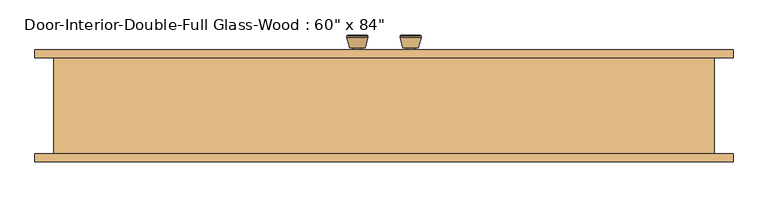
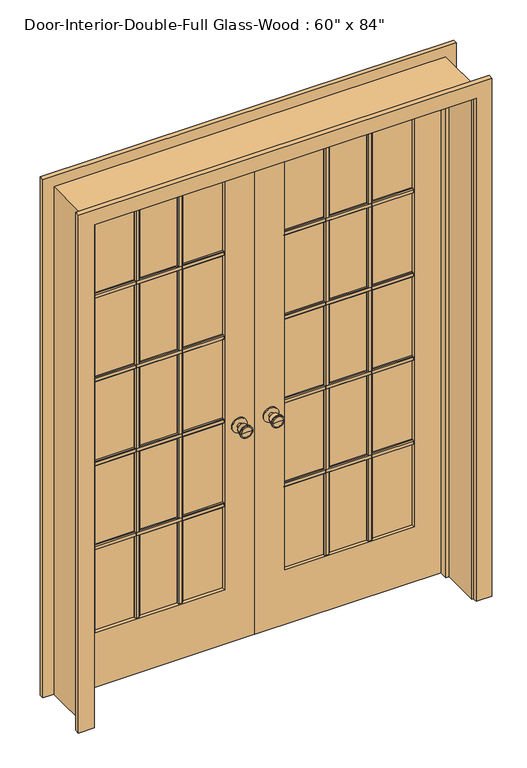
"""IFC4 building model written with IfcOpenShell, lengths in millimetres: door geometry."""

from ifc_helpers import new_model, si_unit, point, frame, frame_2d, origin, place, context, project, spatial, polyline, circle_curve, trimmed, segment, composite_curve, outline, extrude, faceted_brep, source, transform, mapped, element, save
from ifc_brep_helpers import plane_surface, cylinder_surface, revolved_surface, advanced_brep


def door_610bc5f6(model_context):
    return source(origin(), model_context, "Body", "SolidModel", [
        advanced_brep(
        [(-63.5, 117.125, 914.4), (-73.5, 117.125, 914.4), (-53.5, 117.125, 914.4), (-83.9758676, 166.125, 914.4), (-63.5, 166.125, 914.4), (-43.0241324, 166.125, 914.4), (-88.5, 164.2971319, 914.4), (-38.5, 164.2971319, 914.4), (-88.5, 160.8334537, 914.4), (-38.5, 160.8334537, 914.4), (-82.136236, 136.125, 914.4), (-44.863764, 136.125, 914.4), (-73.5, 136.125, 914.4), (-53.5, 136.125, 914.4)],
        [
            (0, 1),
            (1, 2, circle_curve(frame((-63.5, 117.125, 914.4), z_axis=(0.0, -1.0, 0.0), x_axis=(1.0, 0.0, 0.0)), 10.0)),
            (2, 0),
            (2, 1, circle_curve(frame((-63.5, 117.125, 914.4), z_axis=(0.0, -1.0, 0.0), x_axis=(1.0, 0.0, 0.0)), 10.0)),
            (3, 4),
            (4, 5),
            (5, 3, circle_curve(frame((-63.5, 166.125, 914.4), z_axis=(0.0, 1.0, 0.0), x_axis=(1.0, 0.0, 0.0)), 20.4758676)),
            (3, 5, circle_curve(frame((-63.5, 166.125, 914.4), z_axis=(0.0, 1.0, 0.0), x_axis=(1.0, 0.0, 0.0)), 20.4758676)),
            (6, 3),
            (5, 7),
            (7, 6, circle_curve(frame((-63.5, 164.2971319, 914.4), z_axis=(0.0, 1.0, 0.0), x_axis=(1.0, 0.0, 0.0)), 25.0)),
            (6, 7, circle_curve(frame((-63.5, 164.2971319, 914.4), z_axis=(0.0, 1.0, 0.0), x_axis=(1.0, 0.0, 0.0)), 25.0)),
            (8, 6),
            (7, 9),
            (9, 8, circle_curve(frame((-63.5, 160.8334537, 914.4), z_axis=(0.0, 1.0, 0.0), x_axis=(1.0, 0.0, 0.0)), 25.0)),
            (8, 9, circle_curve(frame((-63.5, 160.8334537, 914.4), z_axis=(0.0, 1.0, 0.0), x_axis=(1.0, 0.0, 0.0)), 25.0)),
            (10, 8),
            (9, 11),
            (11, 10, circle_curve(frame((-63.5, 136.125, 914.4), z_axis=(0.0, 1.0, 0.0), x_axis=(1.0, 0.0, 0.0)), 18.636236)),
            (10, 11, circle_curve(frame((-63.5, 136.125, 914.4), z_axis=(0.0, 1.0, 0.0), x_axis=(1.0, 0.0, 0.0)), 18.636236)),
            (12, 10),
            (11, 13),
            (13, 12, circle_curve(frame((-63.5, 136.125, 914.4), z_axis=(0.0, 1.0, 0.0), x_axis=(1.0, 0.0, 0.0)), 10.0)),
            (12, 13, circle_curve(frame((-63.5, 136.125, 914.4), z_axis=(0.0, 1.0, 0.0), x_axis=(1.0, 0.0, 0.0)), 10.0)),
            (1, 12),
            (13, 2),
        ],
        [
            plane_surface(frame((-63.5, 117.125, 914.4), z_axis=(0.0, -1.0, 0.0), x_axis=(1.0, 0.0, 0.0))),
            plane_surface(frame((-63.5, 166.125, 914.4), z_axis=(0.0, 1.0, 0.0), x_axis=(1.0, 0.0, 0.0))),
            revolved_surface(polyline([(-43.0241324, 166.125, 914.4), (-38.5, 164.2971319, 914.4)]), (-63.5, 117.125, 914.4), (0.0, -1.0, 0.0)),
            cylinder_surface(frame((-63.5, 117.125, 914.4), z_axis=(0.0, -1.0, 0.0), x_axis=(1.0, 0.0, 0.0)), 25.0),
            revolved_surface(polyline([(-38.5, 160.8334537, 914.4), (-44.863764, 136.125, 914.4)]), (-63.5, 117.125, 914.4), (0.0, -1.0, 0.0)),
            plane_surface(frame((-63.5, 136.125, 914.4), z_axis=(0.0, -1.0, 0.0), x_axis=(1.0, 0.0, 0.0))),
            cylinder_surface(frame((-63.5, 117.125, 914.4), z_axis=(0.0, -1.0, 0.0), x_axis=(1.0, 0.0, 0.0)), 10.0),
        ],
        [
            (0, [[1, 2, 3]]),
            (0, [[-3, 4, -1]]),
            (1, [[5, 6, 7]]),
            (1, [[-6, -5, 8]]),
            (2, [[9, -7, 10, 11]]),
            (2, [[-10, -8, -9, 12]]),
            (3, [[13, -11, 14, 15]]),
            (3, [[-14, -12, -13, 16]]),
            (4, [[17, -15, 18, 19]]),
            (4, [[-18, -16, -17, 20]]),
            (5, [[21, -19, 22, 23]]),
            (5, [[-22, -20, -21, 24]]),
            (6, [[25, -23, 26, -2]]),
            (6, [[-26, -24, -25, -4]]),
        ],
    ),
        extrude(outline(composite_curve([segment(trimmed(circle_curve(frame_2d((914.4, -63.5)), 30.0), [point((914.4, -33.5))], [point((914.4, -93.5))], False, "CARTESIAN"), True, "CONTINUOUS"), segment(trimmed(circle_curve(frame_2d((914.4, -63.5)), 30.0), [point((914.4, -93.5))], [point((914.4, -33.5))], False, "CARTESIAN"), True, "CONTINUOUS")], self_intersect=False)), frame((0.0, 111.125, 0.0), z_axis=(0.0, 1.0, 0.0), x_axis=(0.0, 0.0, 1.0)), (0.0, 0.0, 1.0), 6.0),
        advanced_brep(
        [(-63.5, 70.2, 914.4), (-53.5, 70.2, 914.4), (-73.5, 70.2, 914.4), (-83.9758676, 21.2, 914.4), (-43.0241324, 21.2, 914.4), (-63.5, 21.2, 914.4), (-88.5, 23.0278681, 914.4), (-38.5, 23.0278681, 914.4), (-88.5, 26.4915463, 914.4), (-38.5, 26.4915463, 914.4), (-82.136236, 51.2, 914.4), (-44.863764, 51.2, 914.4), (-73.5, 51.2, 914.4), (-53.5, 51.2, 914.4)],
        [
            (0, 1),
            (1, 2, circle_curve(frame((-63.5, 70.2, 914.4), z_axis=(0.0, 1.0, 0.0), x_axis=(1.0, 0.0, 0.0)), 10.0)),
            (2, 0),
            (2, 1, circle_curve(frame((-63.5, 70.2, 914.4), z_axis=(0.0, 1.0, 0.0), x_axis=(1.0, 0.0, 0.0)), 10.0)),
            (3, 4, circle_curve(frame((-63.5, 21.2, 914.4), z_axis=(0.0, -1.0, 0.0), x_axis=(1.0, 0.0, 0.0)), 20.4758676)),
            (4, 5),
            (5, 3),
            (4, 3, circle_curve(frame((-63.5, 21.2, 914.4), z_axis=(0.0, -1.0, 0.0), x_axis=(1.0, 0.0, 0.0)), 20.4758676)),
            (6, 7, circle_curve(frame((-63.5, 23.0278681, 914.4), z_axis=(0.0, -1.0, 0.0), x_axis=(1.0, 0.0, 0.0)), 25.0)),
            (7, 4),
            (3, 6),
            (7, 6, circle_curve(frame((-63.5, 23.0278681, 914.4), z_axis=(0.0, -1.0, 0.0), x_axis=(1.0, 0.0, 0.0)), 25.0)),
            (8, 9, circle_curve(frame((-63.5, 26.4915463, 914.4), z_axis=(0.0, -1.0, 0.0), x_axis=(1.0, 0.0, 0.0)), 25.0)),
            (9, 7),
            (6, 8),
            (9, 8, circle_curve(frame((-63.5, 26.4915463, 914.4), z_axis=(0.0, -1.0, 0.0), x_axis=(1.0, 0.0, 0.0)), 25.0)),
            (10, 11, circle_curve(frame((-63.5, 51.2, 914.4), z_axis=(0.0, -1.0, 0.0), x_axis=(1.0, 0.0, 0.0)), 18.636236)),
            (11, 9),
            (8, 10),
            (11, 10, circle_curve(frame((-63.5, 51.2, 914.4), z_axis=(0.0, -1.0, 0.0), x_axis=(1.0, 0.0, 0.0)), 18.636236)),
            (12, 13, circle_curve(frame((-63.5, 51.2, 914.4), z_axis=(0.0, -1.0, 0.0), x_axis=(1.0, 0.0, 0.0)), 10.0)),
            (13, 11),
            (10, 12),
            (13, 12, circle_curve(frame((-63.5, 51.2, 914.4), z_axis=(0.0, -1.0, 0.0), x_axis=(1.0, 0.0, 0.0)), 10.0)),
            (1, 13),
            (12, 2),
        ],
        [
            plane_surface(frame((-63.5, 70.2, 914.4), z_axis=(0.0, 1.0, 0.0), x_axis=(1.0, 0.0, 0.0))),
            plane_surface(frame((-63.5, 21.2, 914.4), z_axis=(0.0, -1.0, 0.0), x_axis=(1.0, 0.0, 0.0))),
            revolved_surface(polyline([(-43.0241324, 21.2, 914.4), (-38.5, 23.0278681, 914.4)]), (-63.5, 70.2, 914.4), (0.0, 1.0, 0.0)),
            cylinder_surface(frame((-63.5, 70.2, 914.4), z_axis=(0.0, 1.0, 0.0), x_axis=(1.0, 0.0, 0.0)), 25.0),
            revolved_surface(polyline([(-38.5, 26.4915463, 914.4), (-44.863764, 51.2, 914.4)]), (-63.5, 70.2, 914.4), (0.0, 1.0, 0.0)),
            plane_surface(frame((-63.5, 51.2, 914.4), z_axis=(0.0, 1.0, 0.0), x_axis=(1.0, 0.0, 0.0))),
            cylinder_surface(frame((-63.5, 70.2, 914.4), z_axis=(0.0, 1.0, 0.0), x_axis=(1.0, 0.0, 0.0)), 10.0),
        ],
        [
            (0, [[1, 2, 3]]),
            (0, [[-3, 4, -1]]),
            (1, [[5, 6, 7]]),
            (1, [[8, -7, -6]]),
            (2, [[9, 10, -5, 11]]),
            (2, [[12, -11, -8, -10]]),
            (3, [[13, 14, -9, 15]]),
            (3, [[16, -15, -12, -14]]),
            (4, [[17, 18, -13, 19]]),
            (4, [[20, -19, -16, -18]]),
            (5, [[21, 22, -17, 23]]),
            (5, [[24, -23, -20, -22]]),
            (6, [[-2, 25, -21, 26]]),
            (6, [[-4, -26, -24, -25]]),
        ],
    ),
        extrude(outline(composite_curve([segment(trimmed(circle_curve(frame_2d((914.4, -63.5)), 30.0), [point((914.4, -33.5))], [point((914.4, -93.5))], False, "CARTESIAN"), True, "CONTINUOUS"), segment(trimmed(circle_curve(frame_2d((914.4, -63.5)), 30.0), [point((914.4, -93.5))], [point((914.4, -33.5))], False, "CARTESIAN"), True, "CONTINUOUS")], self_intersect=False)), frame((0.0, 70.2, 0.0), z_axis=(0.0, 1.0, 0.0), x_axis=(0.0, 0.0, 1.0)), (0.0, 0.0, 1.0), 6.0),
        extrude(outline(polyline([(90.17, 1667.51), (90.17, 1648.46), (83.82, 1648.46), (80.645, 1651.635), (80.645, 1664.335), (83.82, 1667.51), (90.17, 1667.51)])), frame((120.65, 0.0, 0.0), z_axis=(1.0, 0.0, 0.0), x_axis=(0.0, 1.0, 0.0)), (0.0, 0.0, 1.0), 520.7),
        extrude(outline(polyline([(90.17, 1310.9575), (90.17, 1291.9075), (83.82, 1291.9075), (80.645, 1295.0825), (80.645, 1307.7825), (83.82, 1310.9575), (90.17, 1310.9575)])), frame((120.65, 0.0, 0.0), z_axis=(1.0, 0.0, 0.0), x_axis=(0.0, 1.0, 0.0)), (0.0, 0.0, 1.0), 520.7),
        extrude(outline(polyline([(90.17, 954.405), (90.17, 935.355), (83.82, 935.355), (80.645, 938.53), (80.645, 951.23), (83.82, 954.405), (90.17, 954.405)])), frame((120.65, 0.0, 0.0), z_axis=(1.0, 0.0, 0.0), x_axis=(0.0, 1.0, 0.0)), (0.0, 0.0, 1.0), 520.7),
        extrude(outline(polyline([(90.17, 597.8525), (90.17, 578.8025), (83.82, 578.8025), (80.645, 581.9775), (80.645, 594.6775), (83.82, 597.8525), (90.17, 597.8525)])), frame((120.65, 0.0, 0.0), z_axis=(1.0, 0.0, 0.0), x_axis=(0.0, 1.0, 0.0)), (0.0, 0.0, 1.0), 520.7),
        extrude(outline(polyline([(458.2583333, 90.17), (477.3083333, 90.17), (477.3083333, 83.82), (474.1333333, 80.645), (461.4333333, 80.645), (458.2583333, 83.82), (458.2583333, 90.17)])), frame((0.0, 0.0, 231.775), z_axis=(0.0, 0.0, 1.0), x_axis=(1.0, 0.0, 0.0)), (0.0, 0.0, 1.0), 1782.7625),
        extrude(outline(polyline([(284.6916667, 90.17), (303.7416667, 90.17), (303.7416667, 83.82), (300.5666667, 80.645), (287.8666667, 80.645), (284.6916667, 83.82), (284.6916667, 90.17)])), frame((0.0, 0.0, 231.775), z_axis=(0.0, 0.0, 1.0), x_axis=(1.0, 0.0, 0.0)), (0.0, 0.0, 1.0), 1782.7625),
        extrude(outline(polyline([(97.155, 1667.51), (103.505, 1667.51), (106.68, 1664.335), (106.68, 1651.635), (103.505, 1648.46), (97.155, 1648.46), (97.155, 1667.51)])), frame((-641.35, 0.0, 0.0), z_axis=(1.0, 0.0, 0.0), x_axis=(0.0, 1.0, 0.0)), (0.0, 0.0, 1.0), 520.7),
        extrude(outline(polyline([(97.155, 1310.9575), (103.505, 1310.9575), (106.68, 1307.7825), (106.68, 1295.0825), (103.505, 1291.9075), (97.155, 1291.9075), (97.155, 1310.9575)])), frame((-641.35, 0.0, 0.0), z_axis=(1.0, 0.0, 0.0), x_axis=(0.0, 1.0, 0.0)), (0.0, 0.0, 1.0), 520.7),
        extrude(outline(polyline([(97.155, 954.405), (103.505, 954.405), (106.68, 951.23), (106.68, 938.53), (103.505, 935.355), (97.155, 935.355), (97.155, 954.405)])), frame((-641.35, 0.0, 0.0), z_axis=(1.0, 0.0, 0.0), x_axis=(0.0, 1.0, 0.0)), (0.0, 0.0, 1.0), 520.7),
        extrude(outline(polyline([(97.155, 597.8525), (103.505, 597.8525), (106.68, 594.6775), (106.68, 581.9775), (103.505, 578.8025), (97.155, 578.8025), (97.155, 597.8525)])), frame((-641.35, 0.0, 0.0), z_axis=(1.0, 0.0, 0.0), x_axis=(0.0, 1.0, 0.0)), (0.0, 0.0, 1.0), 520.7),
        extrude(outline(polyline([(-303.7416667, 97.155), (-303.7416667, 103.505), (-300.5666667, 106.68), (-287.8666667, 106.68), (-284.6916667, 103.505), (-284.6916667, 97.155), (-303.7416667, 97.155)])), frame((0.0, 0.0, 231.775), z_axis=(0.0, 0.0, 1.0), x_axis=(1.0, 0.0, 0.0)), (0.0, 0.0, 1.0), 1782.7625),
        extrude(outline(polyline([(-477.3083333, 97.155), (-477.3083333, 103.505), (-474.1333333, 106.68), (-461.4333333, 106.68), (-458.2583333, 103.505), (-458.2583333, 97.155), (-477.3083333, 97.155)])), frame((0.0, 0.0, 231.775), z_axis=(0.0, 0.0, 1.0), x_axis=(1.0, 0.0, 0.0)), (0.0, 0.0, 1.0), 1782.7625),
        extrude(outline(polyline([(97.155, 1667.51), (103.505, 1667.51), (106.68, 1664.335), (106.68, 1651.635), (103.505, 1648.46), (97.155, 1648.46), (97.155, 1667.51)])), frame((120.65, 0.0, 0.0), z_axis=(1.0, 0.0, 0.0), x_axis=(0.0, 1.0, 0.0)), (0.0, 0.0, 1.0), 520.7),
        extrude(outline(polyline([(97.155, 1310.9575), (103.505, 1310.9575), (106.68, 1307.7825), (106.68, 1295.0825), (103.505, 1291.9075), (97.155, 1291.9075), (97.155, 1310.9575)])), frame((120.65, 0.0, 0.0), z_axis=(1.0, 0.0, 0.0), x_axis=(0.0, 1.0, 0.0)), (0.0, 0.0, 1.0), 520.7),
        extrude(outline(polyline([(97.155, 954.405), (103.505, 954.405), (106.68, 951.23), (106.68, 938.53), (103.505, 935.355), (97.155, 935.355), (97.155, 954.405)])), frame((120.65, 0.0, 0.0), z_axis=(1.0, 0.0, 0.0), x_axis=(0.0, 1.0, 0.0)), (0.0, 0.0, 1.0), 520.7),
        extrude(outline(polyline([(97.155, 597.8525), (103.505, 597.8525), (106.68, 594.6775), (106.68, 581.9775), (103.505, 578.8025), (97.155, 578.8025), (97.155, 597.8525)])), frame((120.65, 0.0, 0.0), z_axis=(1.0, 0.0, 0.0), x_axis=(0.0, 1.0, 0.0)), (0.0, 0.0, 1.0), 520.7),
        extrude(outline(polyline([(458.2583333, 97.155), (458.2583333, 103.505), (461.4333333, 106.68), (474.1333333, 106.68), (477.3083333, 103.505), (477.3083333, 97.155), (458.2583333, 97.155)])), frame((0.0, 0.0, 231.775), z_axis=(0.0, 0.0, 1.0), x_axis=(1.0, 0.0, 0.0)), (0.0, 0.0, 1.0), 1782.7625),
        extrude(outline(polyline([(284.6916667, 97.155), (284.6916667, 103.505), (287.8666667, 106.68), (300.5666667, 106.68), (303.7416667, 103.505), (303.7416667, 97.155), (284.6916667, 97.155)])), frame((0.0, 0.0, 231.775), z_axis=(0.0, 0.0, 1.0), x_axis=(1.0, 0.0, 0.0)), (0.0, 0.0, 1.0), 1782.7625),
        extrude(outline(polyline([(90.17, 1667.51), (90.17, 1648.46), (83.82, 1648.46), (80.645, 1651.635), (80.645, 1664.335), (83.82, 1667.51), (90.17, 1667.51)])), frame((-641.35, 0.0, 0.0), z_axis=(1.0, 0.0, 0.0), x_axis=(0.0, 1.0, 0.0)), (0.0, 0.0, 1.0), 520.7),
        extrude(outline(polyline([(90.17, 1310.9575), (90.17, 1291.9075), (83.82, 1291.9075), (80.645, 1295.0825), (80.645, 1307.7825), (83.82, 1310.9575), (90.17, 1310.9575)])), frame((-641.35, 0.0, 0.0), z_axis=(1.0, 0.0, 0.0), x_axis=(0.0, 1.0, 0.0)), (0.0, 0.0, 1.0), 520.7),
        extrude(outline(polyline([(90.17, 954.405), (90.17, 935.355), (83.82, 935.355), (80.645, 938.53), (80.645, 951.23), (83.82, 954.405), (90.17, 954.405)])), frame((-641.35, 0.0, 0.0), z_axis=(1.0, 0.0, 0.0), x_axis=(0.0, 1.0, 0.0)), (0.0, 0.0, 1.0), 520.7),
        extrude(outline(polyline([(90.17, 597.8525), (90.17, 578.8025), (83.82, 578.8025), (80.645, 581.9775), (80.645, 594.6775), (83.82, 597.8525), (90.17, 597.8525)])), frame((-641.35, 0.0, 0.0), z_axis=(1.0, 0.0, 0.0), x_axis=(0.0, 1.0, 0.0)), (0.0, 0.0, 1.0), 520.7),
        extrude(outline(polyline([(-303.7416667, 90.17), (-284.6916667, 90.17), (-284.6916667, 83.82), (-287.8666667, 80.645), (-300.5666667, 80.645), (-303.7416667, 83.82), (-303.7416667, 90.17)])), frame((0.0, 0.0, 231.775), z_axis=(0.0, 0.0, 1.0), x_axis=(1.0, 0.0, 0.0)), (0.0, 0.0, 1.0), 1782.7625),
        extrude(outline(polyline([(-477.3083333, 90.17), (-458.2583333, 90.17), (-458.2583333, 83.82), (-461.4333333, 80.645), (-474.1333333, 80.645), (-477.3083333, 83.82), (-477.3083333, 90.17)])), frame((0.0, 0.0, 231.775), z_axis=(0.0, 0.0, 1.0), x_axis=(1.0, 0.0, 0.0)), (0.0, 0.0, 1.0), 1782.7625),
        advanced_brep(
        [(63.5, 70.2, 914.4), (73.5, 70.2, 914.4), (53.5, 70.2, 914.4), (83.9758676, 21.2, 914.4), (63.5, 21.2, 914.4), (43.0241324, 21.2, 914.4), (88.5, 23.0278681, 914.4), (38.5, 23.0278681, 914.4), (88.5, 26.4915463, 914.4), (38.5, 26.4915463, 914.4), (82.136236, 51.2, 914.4), (44.863764, 51.2, 914.4), (73.5, 51.2, 914.4), (53.5, 51.2, 914.4)],
        [
            (0, 1),
            (1, 2, circle_curve(frame((63.5, 70.2, 914.4), z_axis=(0.0, 1.0, 0.0), x_axis=(-1.0, 0.0, 0.0)), 10.0)),
            (2, 0),
            (2, 1, circle_curve(frame((63.5, 70.2, 914.4), z_axis=(0.0, 1.0, 0.0), x_axis=(-1.0, 0.0, 0.0)), 10.0)),
            (3, 4),
            (4, 5),
            (5, 3, circle_curve(frame((63.5, 21.2, 914.4), z_axis=(0.0, -1.0, 0.0), x_axis=(-1.0, 0.0, 0.0)), 20.4758676)),
            (3, 5, circle_curve(frame((63.5, 21.2, 914.4), z_axis=(0.0, -1.0, 0.0), x_axis=(-1.0, 0.0, 0.0)), 20.4758676)),
            (6, 3),
            (5, 7),
            (7, 6, circle_curve(frame((63.5, 23.0278681, 914.4), z_axis=(0.0, -1.0, 0.0), x_axis=(-1.0, 0.0, 0.0)), 25.0)),
            (6, 7, circle_curve(frame((63.5, 23.0278681, 914.4), z_axis=(0.0, -1.0, 0.0), x_axis=(-1.0, 0.0, 0.0)), 25.0)),
            (8, 6),
            (7, 9),
            (9, 8, circle_curve(frame((63.5, 26.4915463, 914.4), z_axis=(0.0, -1.0, 0.0), x_axis=(-1.0, 0.0, 0.0)), 25.0)),
            (8, 9, circle_curve(frame((63.5, 26.4915463, 914.4), z_axis=(0.0, -1.0, 0.0), x_axis=(-1.0, 0.0, 0.0)), 25.0)),
            (10, 8),
            (9, 11),
            (11, 10, circle_curve(frame((63.5, 51.2, 914.4), z_axis=(0.0, -1.0, 0.0), x_axis=(-1.0, 0.0, 0.0)), 18.636236)),
            (10, 11, circle_curve(frame((63.5, 51.2, 914.4), z_axis=(0.0, -1.0, 0.0), x_axis=(-1.0, 0.0, 0.0)), 18.636236)),
            (12, 10),
            (11, 13),
            (13, 12, circle_curve(frame((63.5, 51.2, 914.4), z_axis=(0.0, -1.0, 0.0), x_axis=(-1.0, 0.0, 0.0)), 10.0)),
            (12, 13, circle_curve(frame((63.5, 51.2, 914.4), z_axis=(0.0, -1.0, 0.0), x_axis=(-1.0, 0.0, 0.0)), 10.0)),
            (1, 12),
            (13, 2),
        ],
        [
            plane_surface(frame((63.5, 70.2, 914.4), z_axis=(0.0, 1.0, 0.0), x_axis=(-1.0, 0.0, 0.0))),
            plane_surface(frame((63.5, 21.2, 914.4), z_axis=(0.0, -1.0, 0.0), x_axis=(-1.0, 0.0, 0.0))),
            revolved_surface(polyline([(43.0241324, 21.2, 914.4), (38.5, 23.0278681, 914.4)]), (63.5, 70.2, 914.4), (0.0, 1.0, 0.0)),
            cylinder_surface(frame((63.5, 70.2, 914.4), z_axis=(0.0, 1.0, 0.0), x_axis=(-1.0, 0.0, 0.0)), 25.0),
            revolved_surface(polyline([(38.5, 26.4915463, 914.4), (44.863764, 51.2, 914.4)]), (63.5, 70.2, 914.4), (0.0, 1.0, 0.0)),
            plane_surface(frame((63.5, 51.2, 914.4), z_axis=(0.0, 1.0, 0.0), x_axis=(-1.0, 0.0, 0.0))),
            cylinder_surface(frame((63.5, 70.2, 914.4), z_axis=(0.0, 1.0, 0.0), x_axis=(-1.0, 0.0, 0.0)), 10.0),
        ],
        [
            (0, [[1, 2, 3]]),
            (0, [[-3, 4, -1]]),
            (1, [[5, 6, 7]]),
            (1, [[-6, -5, 8]]),
            (2, [[9, -7, 10, 11]]),
            (2, [[-10, -8, -9, 12]]),
            (3, [[13, -11, 14, 15]]),
            (3, [[-14, -12, -13, 16]]),
            (4, [[17, -15, 18, 19]]),
            (4, [[-18, -16, -17, 20]]),
            (5, [[21, -19, 22, 23]]),
            (5, [[-22, -20, -21, 24]]),
            (6, [[25, -23, 26, -2]]),
            (6, [[-26, -24, -25, -4]]),
        ],
    ),
        extrude(outline(composite_curve([segment(trimmed(circle_curve(frame_2d((914.4, 63.5)), 30.0), [point((914.4, 33.5))], [point((914.4, 93.5))], False, "CARTESIAN"), True, "CONTINUOUS"), segment(trimmed(circle_curve(frame_2d((914.4, 63.5)), 30.0), [point((914.4, 93.5))], [point((914.4, 33.5))], False, "CARTESIAN"), True, "CONTINUOUS")], self_intersect=False)), frame((0.0, 70.2, 0.0), z_axis=(0.0, 1.0, 0.0), x_axis=(0.0, 0.0, 1.0)), (0.0, 0.0, 1.0), 6.0),
        advanced_brep(
        [(63.5, 117.125, 914.4), (53.5, 117.125, 914.4), (73.5, 117.125, 914.4), (83.9758676, 166.125, 914.4), (43.0241324, 166.125, 914.4), (63.5, 166.125, 914.4), (88.5, 164.2971319, 914.4), (38.5, 164.2971319, 914.4), (88.5, 160.8334537, 914.4), (38.5, 160.8334537, 914.4), (82.136236, 136.125, 914.4), (44.863764, 136.125, 914.4), (73.5, 136.125, 914.4), (53.5, 136.125, 914.4)],
        [
            (0, 1),
            (1, 2, circle_curve(frame((63.5, 117.125, 914.4), z_axis=(0.0, -1.0, 0.0), x_axis=(-1.0, 0.0, 0.0)), 10.0)),
            (2, 0),
            (2, 1, circle_curve(frame((63.5, 117.125, 914.4), z_axis=(0.0, -1.0, 0.0), x_axis=(-1.0, 0.0, 0.0)), 10.0)),
            (3, 4, circle_curve(frame((63.5, 166.125, 914.4), z_axis=(0.0, 1.0, 0.0), x_axis=(-1.0, 0.0, 0.0)), 20.4758676)),
            (4, 5),
            (5, 3),
            (4, 3, circle_curve(frame((63.5, 166.125, 914.4), z_axis=(0.0, 1.0, 0.0), x_axis=(-1.0, 0.0, 0.0)), 20.4758676)),
            (6, 7, circle_curve(frame((63.5, 164.2971319, 914.4), z_axis=(0.0, 1.0, 0.0), x_axis=(-1.0, 0.0, 0.0)), 25.0)),
            (7, 4),
            (3, 6),
            (7, 6, circle_curve(frame((63.5, 164.2971319, 914.4), z_axis=(0.0, 1.0, 0.0), x_axis=(-1.0, 0.0, 0.0)), 25.0)),
            (8, 9, circle_curve(frame((63.5, 160.8334537, 914.4), z_axis=(0.0, 1.0, 0.0), x_axis=(-1.0, 0.0, 0.0)), 25.0)),
            (9, 7),
            (6, 8),
            (9, 8, circle_curve(frame((63.5, 160.8334537, 914.4), z_axis=(0.0, 1.0, 0.0), x_axis=(-1.0, 0.0, 0.0)), 25.0)),
            (10, 11, circle_curve(frame((63.5, 136.125, 914.4), z_axis=(0.0, 1.0, 0.0), x_axis=(-1.0, 0.0, 0.0)), 18.636236)),
            (11, 9),
            (8, 10),
            (11, 10, circle_curve(frame((63.5, 136.125, 914.4), z_axis=(0.0, 1.0, 0.0), x_axis=(-1.0, 0.0, 0.0)), 18.636236)),
            (12, 13, circle_curve(frame((63.5, 136.125, 914.4), z_axis=(0.0, 1.0, 0.0), x_axis=(-1.0, 0.0, 0.0)), 10.0)),
            (13, 11),
            (10, 12),
            (13, 12, circle_curve(frame((63.5, 136.125, 914.4), z_axis=(0.0, 1.0, 0.0), x_axis=(-1.0, 0.0, 0.0)), 10.0)),
            (1, 13),
            (12, 2),
        ],
        [
            plane_surface(frame((63.5, 117.125, 914.4), z_axis=(0.0, -1.0, 0.0), x_axis=(-1.0, 0.0, 0.0))),
            plane_surface(frame((63.5, 166.125, 914.4), z_axis=(0.0, 1.0, 0.0), x_axis=(-1.0, 0.0, 0.0))),
            revolved_surface(polyline([(43.0241324, 166.125, 914.4), (38.5, 164.2971319, 914.4)]), (63.5, 117.125, 914.4), (0.0, -1.0, 0.0)),
            cylinder_surface(frame((63.5, 117.125, 914.4), z_axis=(0.0, -1.0, 0.0), x_axis=(-1.0, 0.0, 0.0)), 25.0),
            revolved_surface(polyline([(38.5, 160.8334537, 914.4), (44.863764, 136.125, 914.4)]), (63.5, 117.125, 914.4), (0.0, -1.0, 0.0)),
            plane_surface(frame((63.5, 136.125, 914.4), z_axis=(0.0, -1.0, 0.0), x_axis=(-1.0, 0.0, 0.0))),
            cylinder_surface(frame((63.5, 117.125, 914.4), z_axis=(0.0, -1.0, 0.0), x_axis=(-1.0, 0.0, 0.0)), 10.0),
        ],
        [
            (0, [[1, 2, 3]]),
            (0, [[-3, 4, -1]]),
            (1, [[5, 6, 7]]),
            (1, [[8, -7, -6]]),
            (2, [[9, 10, -5, 11]]),
            (2, [[12, -11, -8, -10]]),
            (3, [[13, 14, -9, 15]]),
            (3, [[16, -15, -12, -14]]),
            (4, [[17, 18, -13, 19]]),
            (4, [[20, -19, -16, -18]]),
            (5, [[21, 22, -17, 23]]),
            (5, [[24, -23, -20, -22]]),
            (6, [[-2, 25, -21, 26]]),
            (6, [[-4, -26, -24, -25]]),
        ],
    ),
        extrude(outline(composite_curve([segment(trimmed(circle_curve(frame_2d((914.4, 63.5)), 30.0), [point((914.4, 33.5))], [point((914.4, 93.5))], False, "CARTESIAN"), True, "CONTINUOUS"), segment(trimmed(circle_curve(frame_2d((914.4, 63.5)), 30.0), [point((914.4, 93.5))], [point((914.4, 33.5))], False, "CARTESIAN"), True, "CONTINUOUS")], self_intersect=False)), frame((0.0, 111.125, 0.0), z_axis=(0.0, 1.0, 0.0), x_axis=(0.0, 0.0, 1.0)), (0.0, 0.0, 1.0), 6.0),
        extrude(outline(polyline([(0.0, 768.35), (0.0, 831.85), (2203.45, 831.85), (2203.45, -831.85), (0.0, -831.85), (0.0, -768.35), (2139.95, -768.35), (2139.95, 768.35), (0.0, 768.35)])), frame((0.0, -136.525, 0.0), z_axis=(0.0, 1.0, 0.0), x_axis=(0.0, 0.0, 1.0)), (0.0, 0.0, 1.0), 19.05),
        extrude(outline(polyline([(0.0, 768.35), (0.0, 831.85), (2203.45, 831.85), (2203.45, -831.85), (0.0, -831.85), (0.0, -768.35), (2139.95, -768.35), (2139.95, 768.35), (0.0, 768.35)])), frame((0.0, 111.125, 0.0), z_axis=(0.0, 1.0, 0.0), x_axis=(0.0, 0.0, 1.0)), (0.0, 0.0, 1.0), 19.05),
        faceted_brep([(787.4, 111.125, 0.0), (787.4, -117.475, 0.0), (762.0, -117.475, 0.0), (762.0, 41.275, 0.0), (749.3, 41.275, 0.0), (749.3, 76.2, 0.0), (762.0, 76.2, 0.0), (762.0, 111.125, 0.0), (787.4, 111.125, 2159.0), (787.4, -117.475, 2159.0), (-787.4, -117.475, 2159.0), (-787.4, -117.475, 0.0), (-762.0, -117.475, 0.0), (-762.0, -117.475, 2133.6), (762.0, -117.475, 2133.6), (762.0, 41.275, 2133.6), (-762.0, 41.275, 2133.6), (-762.0, 41.275, 0.0), (-749.3, 41.275, 0.0), (-749.3, 41.275, 2120.9), (749.3, 41.275, 2120.9), (749.3, 76.2, 2120.9), (1.5875, 76.2, 2120.9), (-1.6019111, 76.2, 2120.9), (-749.3, 76.2, 2120.9), (-749.3, 76.2, 0.0), (-762.0, 76.2, 0.0), (-762.0, 76.2, 2133.6), (-1.6019111, 76.2, 2133.6), (1.5875, 76.2, 2133.6), (762.0, 76.2, 2133.6), (762.0, 111.125, 2133.6), (1.5875, 111.125, 2133.6), (-1.6019111, 111.125, 2133.6), (-762.0, 111.125, 2133.6), (-762.0, 111.125, 0.0), (-787.4, 111.125, 0.0), (-787.4, 111.125, 2159.0)], [[[0, 1, 2, 3, 4, 5, 6, 7]], [[1, 0, 8, 9]], [[2, 1, 9, 10, 11, 12, 13, 14]], [[3, 2, 14, 15]], [[4, 3, 15, 16, 17, 18, 19, 20]], [[5, 4, 20, 21]], [[6, 5, 21, 22, 23, 24, 25, 26, 27, 28, 29, 30]], [[7, 6, 30, 31]], [[0, 7, 31, 32, 33, 34, 35, 36, 37, 8]], [[9, 8, 37, 10]], [[14, 13, 16, 15]], [[20, 19, 24, 23, 22, 21]], [[31, 30, 29, 28, 27, 34, 33, 32]], [[12, 11, 36, 35, 26, 25, 18, 17]], [[11, 10, 37, 36]], [[13, 12, 17, 16]], [[19, 18, 25, 24]], [[27, 26, 35, 34]]]),
        extrude(outline(polyline([(2133.6, -762.0), (0.0, -762.0), (0.0, -1.6019111), (2133.6, -1.6019111), (2133.6, -762.0)]), holes=[polyline([(231.775, -641.35), (2014.5375, -641.35), (2014.5375, -120.65), (231.775, -120.65), (231.775, -641.35)])]), frame((0.0, 76.2, 0.0), z_axis=(0.0, 1.0, 0.0), x_axis=(0.0, 0.0, 1.0)), (0.0, 0.0, 1.0), 34.925),
        extrude(outline(polyline([(0.0, 762.0), (2133.6, 762.0), (2133.6, 1.5875), (0.0, 1.5875), (0.0, 762.0)]), holes=[polyline([(2014.5375, 120.65), (2014.5375, 641.35), (231.775, 641.35), (231.775, 120.65), (2014.5375, 120.65)])]), frame((0.0, 76.2, 0.0), z_axis=(0.0, 1.0, 0.0), x_axis=(0.0, 0.0, 1.0)), (0.0, 0.0, 1.0), 34.925),
        extrude(outline(polyline([(641.35, 90.17), (120.65, 90.17), (120.65, 97.155), (641.35, 97.155), (641.35, 90.17)])), frame((0.0, 0.0, 231.775), z_axis=(0.0, 0.0, 1.0), x_axis=(1.0, 0.0, 0.0)), (0.0, 0.0, 1.0), 1782.7625),
        extrude(outline(polyline([(-120.65, 90.17), (-641.35, 90.17), (-641.35, 97.155), (-120.65, 97.155), (-120.65, 90.17)])), frame((0.0, 0.0, 231.775), z_axis=(0.0, 0.0, 1.0), x_axis=(1.0, 0.0, 0.0)), (0.0, 0.0, 1.0), 1782.7625),
    ])


if __name__ == "__main__":
    model = new_model("IFC4")
    model_context = context("Model", 3, world=origin())
    ifc_project = project(units=[si_unit("LENGTHUNIT", "METRE", prefix="MILLI")], contexts=[model_context])
    site = spatial("IfcSite", under=ifc_project)
    building = spatial("IfcBuilding", under=site)
    placement = place(None, origin())
    door_shape = door_610bc5f6(model_context)
    element("IfcDoor", 1, ObjectType="Door-Interior-Double-Full Glass-Wood : 60\" x 84\"", at=placement, inside=building, context=model_context, shape_type="MappedRepresentation", body=[
        mapped(door_shape, transform((0.0, 0.0, 0.0), x_axis=(1.0, 0.0, 0.0), y_axis=(0.0, 1.0, 0.0), z_axis=(0.0, 0.0, 1.0))),
    ])
    save(model, "model.ifc")

# Revit data of these elements
# Type "Door-Interior-Double-Full Glass-Wood : 60\" x 84\""
#   Type Mark = "8"
#   Assembly Code = "C1020300"
#   Analytic Construction = "French door, wood frame with single glass"
#   Top Rail = 0' - 4 11/16"
#   Thickness = 0' - 1 3/8"
#   Thermal Resistance (R) = 1.0696 (h·ft²·°F)/BTU
#   Swing Angle [instance default] = 90.00°
#   Stiles = 0' - 4 3/4"
#   Rough Width = 5' - 2"
#   Rough Height = 7' - 1"
#   Panel Width = 2' - 6"
#   Height = 7' - 0"
#   Width = 5' - 0"
#   Heat Transfer Coefficient (U) = 0.9350 BTU/(h·ft²·°F)
#   Bottom Rail = 0' - 9 1/8"
#   Show Grill [instance default] = yes
#   Trim Material = Cherry
#   Panel Material = Cherry
#   Frame Material = Cherry
#   Door Handle Material = Aluminum
#   Visual Light Transmittance = 0
#   Solar Heat Gain Coefficient = 0
#   Wall Closure = (empty or 0)
#   Function = (empty or 0)
# Element 1 (IfcDoor, "Door-Interior-Double-Full Glass-Wood : 60\" x 84\"")
#   Materials on its faces: "Cherry", "Aluminum", "Glass"
# Materials
#   "Cherry": class "Wood", colour RGB 226 177 128, transparency 0, Description = "Prunus Serotina", Cost = 0
#   "Aluminum": class "Metal", colour RGB 247 247 247, transparency 0, Description = "Aluminum 6061", Cost = 0
#   "Glass": class "Glass", colour RGB 0 128 192, transparency 0.75, Description = "Soda Lime Glass", Cost = 0
